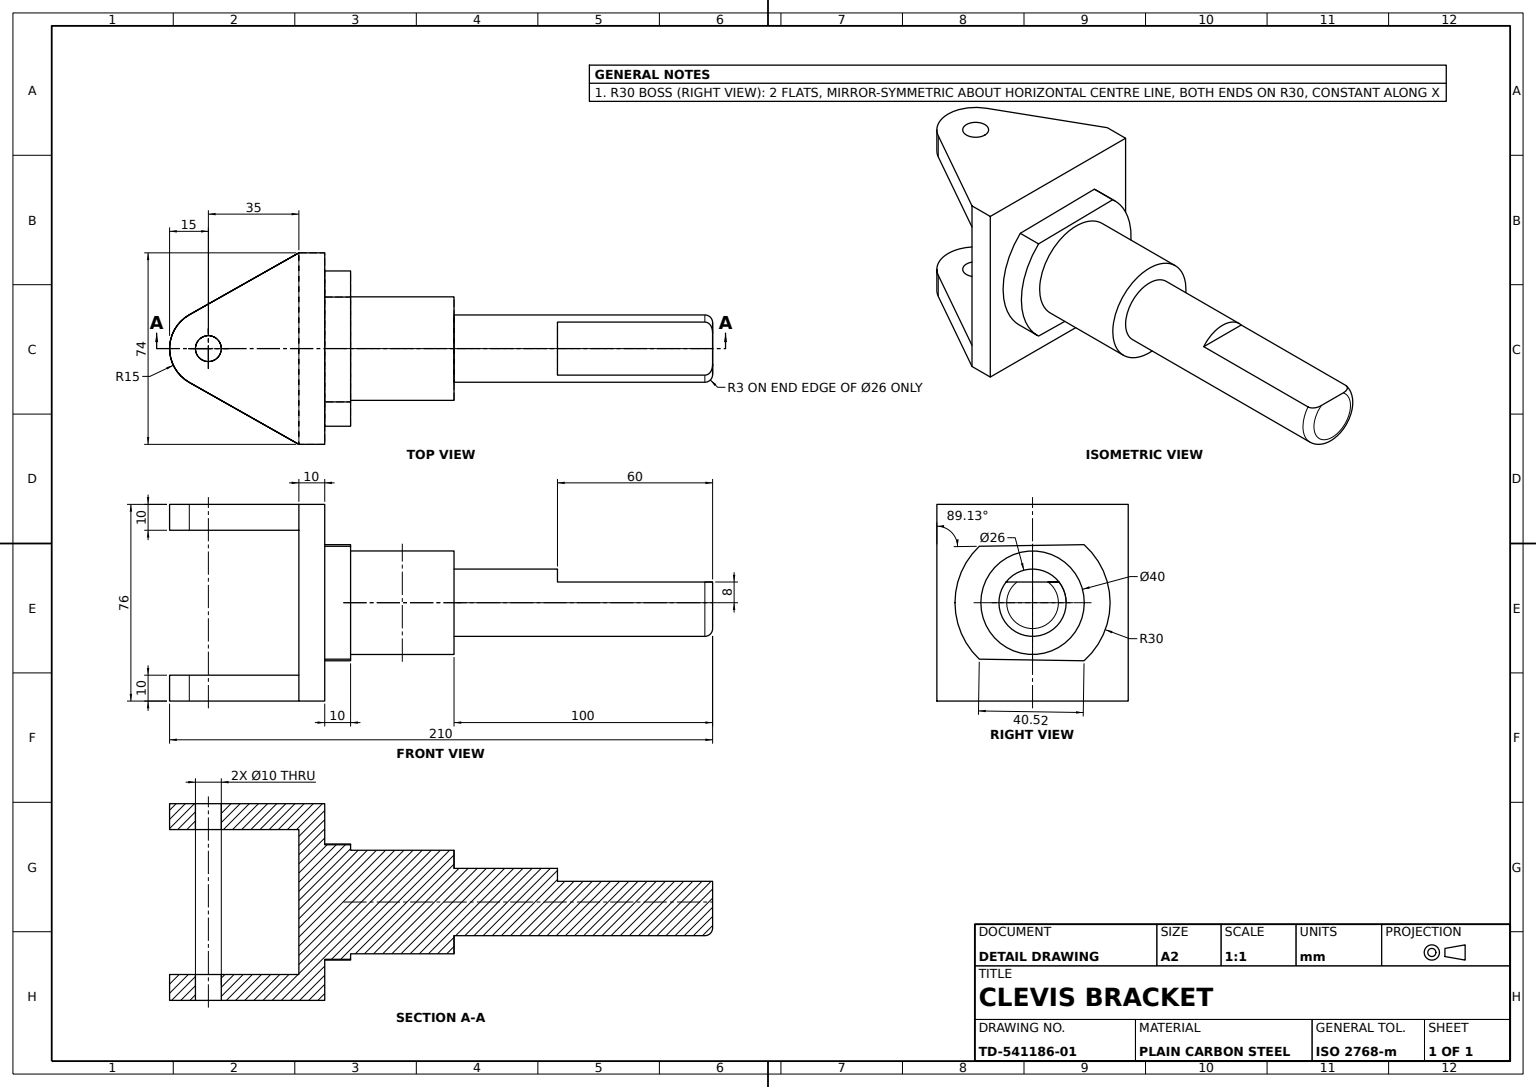
from build123d import *

# Parameters (mm, degrees)
BASE_PLATE_SKETCH_W    = 74
BASE_PLATE_SKETCH_H    = 76
BASE_PLATE_DEPTH       = 10
FLANGE_EAR_A_SKETCH_R  = 5
FLANGE_EAR_A_DEPTH     = 10
FLANGE_START           = -10
FLANGE_EAR_B_SKETCH_R  = 5
FLANGE_EAR_B_DEPTH     = 10
TRANSITION_BOSS_DEPTH  = 10
HUB_40_SKETCH_R        = 20
HUB_40_DEPTH           = 40
SHAFT_26_SKETCH_R      = 13
SHAFT_26_DEPTH         = 100
SHAFT_START            = -60
SHAFT_FLAT_CUT_DEPTH   = 60
SHAFT_EDGE_FILLET_R3_R = 3


with BuildPart() as part:
    # Base Plate Sketch → Base Plate (new body)
    with BuildSketch(Plane.XY):
        Rectangle(BASE_PLATE_SKETCH_W, BASE_PLATE_SKETCH_H)
    extrude(amount=BASE_PLATE_DEPTH)

    # Flange Ear A Sketch → Flange Ear A (add)
    with BuildSketch(Plane(origin=(0, 38, 0), x_dir=(1, 0, 0), z_dir=(0, 1, 0))):
        with BuildLine():
            Line((-37, -10), (-13.060137394, -52.377859531))
            ThreePointArc((-13.060137394, -52.377859531), (0, -60), (13.060137394, -52.377859531))
            Line((13.060137394, -52.377859531), (37, -10))
            Line((37, -10), (-37, -10))
        make_face()
        with Locations(Location((0, -45, 0), (0, 0, 270))):
            Circle(FLANGE_EAR_A_SKETCH_R, mode=Mode.SUBTRACT)
    extrude(amount=-FLANGE_EAR_A_DEPTH)

    # Flange Ear B Sketch → Flange Ear B (add)
    with BuildSketch(Plane.XZ.offset(38).offset(FLANGE_START)):
        with BuildLine():
            Line((-37, 10), (-13.060137394, 52.377859531))
            ThreePointArc((-13.060137394, 52.377859531), (0, 60), (13.060137394, 52.377859531))
            Line((13.060137394, 52.377859531), (37, 10))
            Line((37, 10), (-37, 10))
        make_face()
        with Locations(Location((0, 45, 0), (0, 0, 90))):
            Circle(FLANGE_EAR_B_SKETCH_R, mode=Mode.SUBTRACT)
    extrude(amount=FLANGE_EAR_B_DEPTH)

    # Transition Boss Sketch → Transition Boss (add)
    with BuildSketch(Plane(origin=(0, 0, 0), x_dir=(-1, 0, 0), z_dir=(0, 0, -1))):
        with BuildLine():
            Line((19.921474427, 22.430667771), (-20.596234674, 21.812728331))
            ThreePointArc((-20.596234674, 21.812728331), (-22.10962434, 20.277191904), (-23.508824666, 18.636930081))
            ThreePointArc((-23.508824666, 18.636930081), (-30, 0), (-23.508824666, -18.636930081))
            ThreePointArc((-23.508824666, -18.636930081), (-22.10962434, -20.277191904), (-20.596234674, -21.812728331))
            Line((-20.596234674, -21.812728331), (19.921474427, -22.430667771))
            ThreePointArc((19.921474427, -22.430667771), (21.797840059, -20.611990897), (23.508824666, -18.636930081))
            ThreePointArc((23.508824666, -18.636930081), (30, 0), (23.508824666, 18.636930081))
            ThreePointArc((23.508824666, 18.636930081), (21.797840059, 20.611990897), (19.921474427, 22.430667771))
        make_face()
    extrude(amount=TRANSITION_BOSS_DEPTH)

    # Hub _40 Sketch → Hub _40 (add)
    with BuildSketch(Plane(origin=(0, 0, -10), x_dir=(-1, 0, 0), z_dir=(0, 0, -1))):
        Circle(HUB_40_SKETCH_R)
    extrude(amount=HUB_40_DEPTH)

    # Shaft _26 Sketch → Shaft _26 (add)
    with BuildSketch(Plane(origin=(0, 0, -50), x_dir=(-1, 0, 0), z_dir=(0, 0, -1))):
        Circle(SHAFT_26_SKETCH_R)
    extrude(amount=SHAFT_26_DEPTH)

    # Shaft Flat Sketch → Shaft Flat Cut (cut)
    with BuildSketch(Plane(origin=(0, 0, -150), x_dir=(-1, 0, 0), z_dir=(0, 0, -1)).offset(SHAFT_START)):
        with BuildLine():
            Line((-10.246950766, 8), (10.246950766, 8))
            ThreePointArc((10.246950766, 8), (0, 13), (-10.246950766, 8))
        make_face()
    extrude(amount=SHAFT_FLAT_CUT_DEPTH, mode=Mode.SUBTRACT)

    # Shaft Edge Fillet R3
    shaft_edge_fillet_r3_edges = [part.edges().sort_by_distance(p)[0] for p in [
        (4.230226947, -12.292484695, -150),
    ]]
    fillet(shaft_edge_fillet_r3_edges, radius=SHAFT_EDGE_FILLET_R3_R)


solid = part.part
